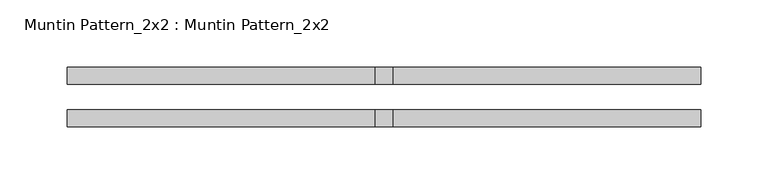
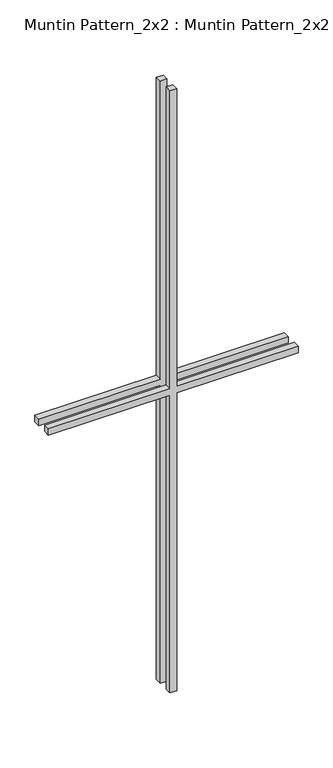
"""IFC4 building model written with IfcOpenShell, lengths in millimetres: proxy geometry, Muntin Pattern_2x2 : Muntin Pattern_2x2."""

from ifc_helpers import new_model, si_unit, frame, origin, place, context, project, spatial, polyline, outline, extrude, source, transform, mapped, element, save


def muntin_pattern_2x2_muntin_pattern_2x2_877df4e9(model_context):
    return source(origin(), model_context, "Body", "SweptSolid", [
        extrude(outline(polyline([(609.6, -6.35), (609.6, -236.5375), (596.9, -236.5375), (596.9, -6.35), (0.0, -6.35), (0.0, 6.35), (596.9, 6.35), (596.9, 236.5375), (609.6, 236.5375), (609.6, 6.35), (1206.5, 6.35), (1206.5, -6.35), (609.6, -6.35)])), frame((0.0, -22.225, 0.0), z_axis=(0.0, 1.0, 0.0), x_axis=(0.0, 0.0, 1.0)), (0.0, 0.0, 1.0), 12.7),
        extrude(outline(polyline([(609.6, -6.35), (609.6, -236.5375), (596.9, -236.5375), (596.9, -6.35), (0.0, -6.35), (0.0, 6.35), (596.9, 6.35), (596.9, 236.5375), (609.6, 236.5375), (609.6, 6.35), (1206.5, 6.35), (1206.5, -6.35), (609.6, -6.35)])), frame((0.0, 9.525, 0.0), z_axis=(0.0, 1.0, 0.0), x_axis=(0.0, 0.0, 1.0)), (0.0, 0.0, 1.0), 12.7),
    ])


if __name__ == "__main__":
    model = new_model("IFC4")
    model_context = context("Model", 3, world=origin())
    ifc_project = project(units=[si_unit("LENGTHUNIT", "METRE", prefix="MILLI")], contexts=[model_context])
    site = spatial("IfcSite", under=ifc_project)
    building = spatial("IfcBuilding", under=site)
    placement = place(None, origin())
    muntin_pattern_2x2_muntin_pattern_2x2_shape = muntin_pattern_2x2_muntin_pattern_2x2_877df4e9(model_context)
    element("IfcBuildingElementProxy", 1, Name="Muntin Pattern_2x2 : Muntin Pattern_2x2", ObjectType="Muntin Pattern_2x2 : Muntin Pattern_2x2", at=placement, inside=building, context=model_context, shape_type="MappedRepresentation", body=[
        mapped(muntin_pattern_2x2_muntin_pattern_2x2_shape, transform((0.0, 0.0, 0.0), x_axis=(1.0, 0.0, 0.0), y_axis=(0.0, 1.0, 0.0), z_axis=(0.0, 0.0, 1.0))),
    ])
    save(model, "model.ifc")

# Revit data of these elements
# Type "Muntin Pattern_2x2 : Muntin Pattern_2x2"
#   Width [instance default] = 4' - 0"
#   Thickness = 0' - 0 1/2"
#   Height [instance default] = 4' - 0"
#   Distance = 0' - 0 3/4"
#   Interior Material [instance default] = none
#   Exterior Material [instance default] = none
#   Default Elevation = 0
# Element 1 (IfcBuildingElementProxy, "Muntin Pattern_2x2 : Muntin Pattern_2x2")
#   Width = 1' - 6 5/8"
#   Height = 3' - 11 1/2"
#   Interior Material = Wood - Stained
#   Exterior Material = Clad - White
#   Materials on its faces: "Clad - White", "Wood - Stained"
# Materials
#   "Clad - White": class "Wood", colour RGB 242 242 238, transparency 0, Cost = 0
#   "Wood - Stained": class "Wood", colour RGB 224 178 126, transparency 0, Cost = 0
